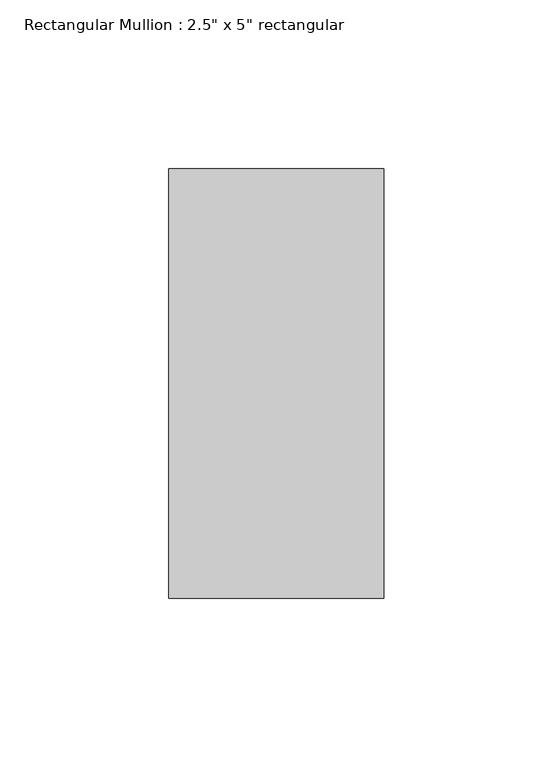
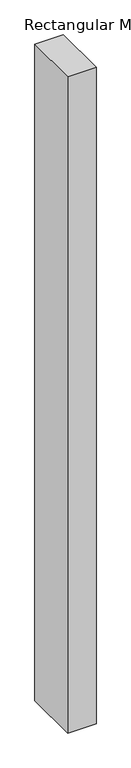
"""IFC4 building model written with IfcOpenShell, lengths in millimetres: member geometry."""

from ifc_helpers import new_model, si_unit, frame, origin, place, context, project, spatial, polyline, outline, extrude, source, transform, mapped, element, save


def member_e254c550(model_context):
    return source(origin(), model_context, "Body", "SweptSolid", [
        extrude(outline(polyline([(31.75, 63.5), (31.75, -63.5), (-31.75, -63.5), (-31.75, 63.5), (31.75, 63.5)])), frame((0.0, 0.0, -1553.5106693), z_axis=(0.0, 0.0, 1.0), x_axis=(1.0, 0.0, 0.0)), (0.0, 0.0, 1.0), 1553.5106693),
    ])


if __name__ == "__main__":
    model = new_model("IFC4")
    model_context = context("Model", 3, world=origin())
    ifc_project = project(units=[si_unit("LENGTHUNIT", "METRE", prefix="MILLI")], contexts=[model_context])
    site = spatial("IfcSite", under=ifc_project)
    building = spatial("IfcBuilding", under=site)
    placement = place(None, origin())
    member_shape = member_e254c550(model_context)
    element("IfcMember", 1, ObjectType="Rectangular Mullion : 2.5\" x 5\" rectangular", at=placement, inside=building, context=model_context, shape_type="MappedRepresentation", body=[
        mapped(member_shape, transform((0.0, 0.0, 0.0), x_axis=(1.0, 0.0, 0.0), y_axis=(0.0, 1.0, 0.0), z_axis=(0.0, 0.0, 1.0))),
    ])
    save(model, "model.ifc")

# Revit data of these elements
# Type "Rectangular Mullion : 2.5\" x 5\" rectangular"
#   built-in parameter 1007304 = 0.416667 (stored number, unit not read)
#   built-in parameter 1007301 = 0.104167 (stored number, unit not read)
#   built-in parameter 1007300 = 0.104167 (stored number, unit not read)
# Element 1 (IfcMember, "Rectangular Mullion : 2.5\" x 5\" rectangular")
#   Materials on its faces: "Aluminum"
# Materials
#   "Aluminum": class "Metal", colour RGB 247 247 247, transparency 0, Description = "Aluminum 6061", Cost = 0
